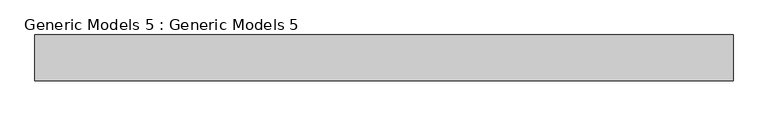
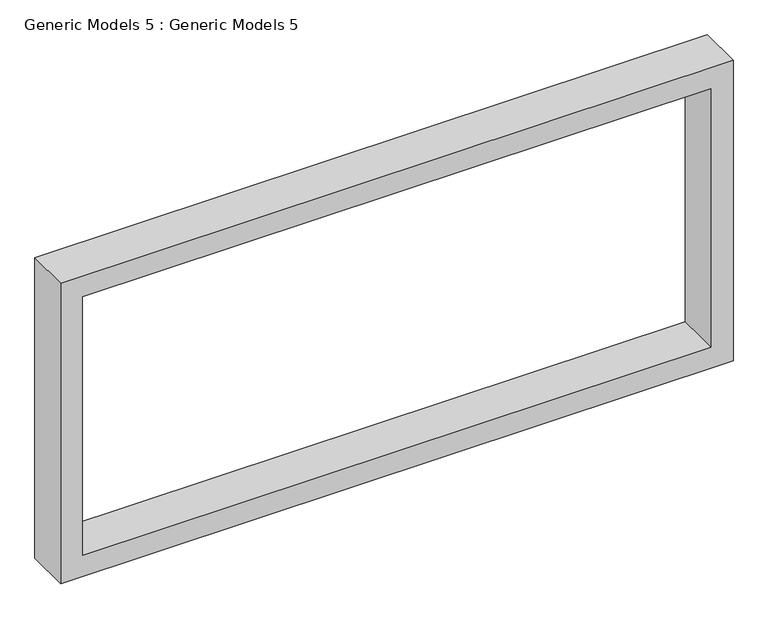
"""IFC4 building model written with IfcOpenShell, lengths in millimetres: proxy geometry, Generic Models 5 : Generic Models 5."""

from ifc_helpers import new_model, si_unit, frame, origin, place, context, project, spatial, polyline, outline, extrude, source, transform, mapped, element, save


def generic_models_5_generic_models_5_57bc8fc0(model_context):
    return source(origin(), model_context, "Body", "SweptSolid", [
        extrude(outline(polyline([(6096.0, -576.2824081), (6096.0, -7510.4824081), (2819.4, -7510.4824081), (2819.4, -576.2824081), (6096.0, -576.2824081)]), holes=[polyline([(5867.4, -804.8824081), (3048.0, -804.8824081), (3048.0, -7281.8824081), (5867.4, -7281.8824081), (5867.4, -804.8824081)])]), frame((0.0, 3743.4444012, 0.0), z_axis=(0.0, 1.0, 0.0), x_axis=(0.0, 0.0, 1.0)), (0.0, 0.0, 1.0), 457.2),
    ])


if __name__ == "__main__":
    model = new_model("IFC4")
    model_context = context("Model", 3, world=origin())
    ifc_project = project(units=[si_unit("LENGTHUNIT", "METRE", prefix="MILLI")], contexts=[model_context])
    site = spatial("IfcSite", under=ifc_project)
    building = spatial("IfcBuilding", under=site)
    placement = place(None, origin())
    generic_models_5_generic_models_5_shape = generic_models_5_generic_models_5_57bc8fc0(model_context)
    element("IfcBuildingElementProxy", 1, Name="Generic Models 5 : Generic Models 5", ObjectType="Generic Models 5 : Generic Models 5", at=placement, inside=building, context=model_context, shape_type="MappedRepresentation", body=[
        mapped(generic_models_5_generic_models_5_shape, transform((0.0, 0.0, 0.0), x_axis=(1.0, 0.0, 0.0), y_axis=(0.0, 1.0, 0.0), z_axis=(0.0, 0.0, 1.0))),
    ])
    save(model, "model.ifc")
